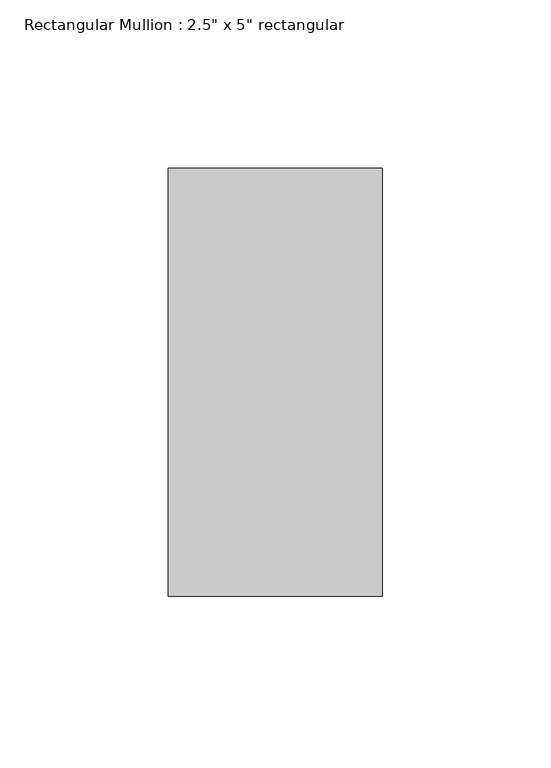
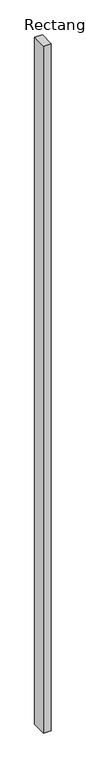
"""IFC4 building model written with IfcOpenShell, lengths in millimetres: member geometry."""

from ifc_helpers import new_model, si_unit, frame, origin, place, context, project, spatial, polyline, outline, extrude, source, transform, mapped, element, save


def member_ecd02cc6(model_context):
    return source(origin(), model_context, "Body", "SweptSolid", [
        extrude(outline(polyline([(31.75, 63.5), (31.75, -63.5), (-31.75, -63.5), (-31.75, 63.5), (31.75, 63.5)])), frame((0.0, 0.0, -6011.7116741), z_axis=(0.0, 0.0, 1.0), x_axis=(1.0, 0.0, 0.0)), (0.0, 0.0, 1.0), 6011.7116741),
    ])


if __name__ == "__main__":
    model = new_model("IFC4")
    model_context = context("Model", 3, world=origin())
    ifc_project = project(units=[si_unit("LENGTHUNIT", "METRE", prefix="MILLI")], contexts=[model_context])
    site = spatial("IfcSite", under=ifc_project)
    building = spatial("IfcBuilding", under=site)
    placement = place(None, origin())
    member_shape = member_ecd02cc6(model_context)
    element("IfcMember", 1, ObjectType="Rectangular Mullion : 2.5\" x 5\" rectangular", at=placement, inside=building, context=model_context, shape_type="MappedRepresentation", body=[
        mapped(member_shape, transform((0.0, 0.0, 0.0), x_axis=(1.0, 0.0, 0.0), y_axis=(0.0, 1.0, 0.0), z_axis=(0.0, 0.0, 1.0))),
    ])
    save(model, "model.ifc")

# Revit data of these elements
# Type "Rectangular Mullion : 2.5\" x 5\" rectangular"
#   built-in parameter 1007304 = 0.416667 (stored number, unit not read)
#   built-in parameter 1007301 = 0.104167 (stored number, unit not read)
#   built-in parameter 1007300 = 0.104167 (stored number, unit not read)
# Element 1 (IfcMember, "Rectangular Mullion : 2.5\" x 5\" rectangular")
#   Materials on its faces: "Iron, Ductile"
# Materials
#   "Iron, Ductile": class "Metal", colour RGB 0 0 0, transparency 0, Description = "Ductile cast iron", Cost = 0
